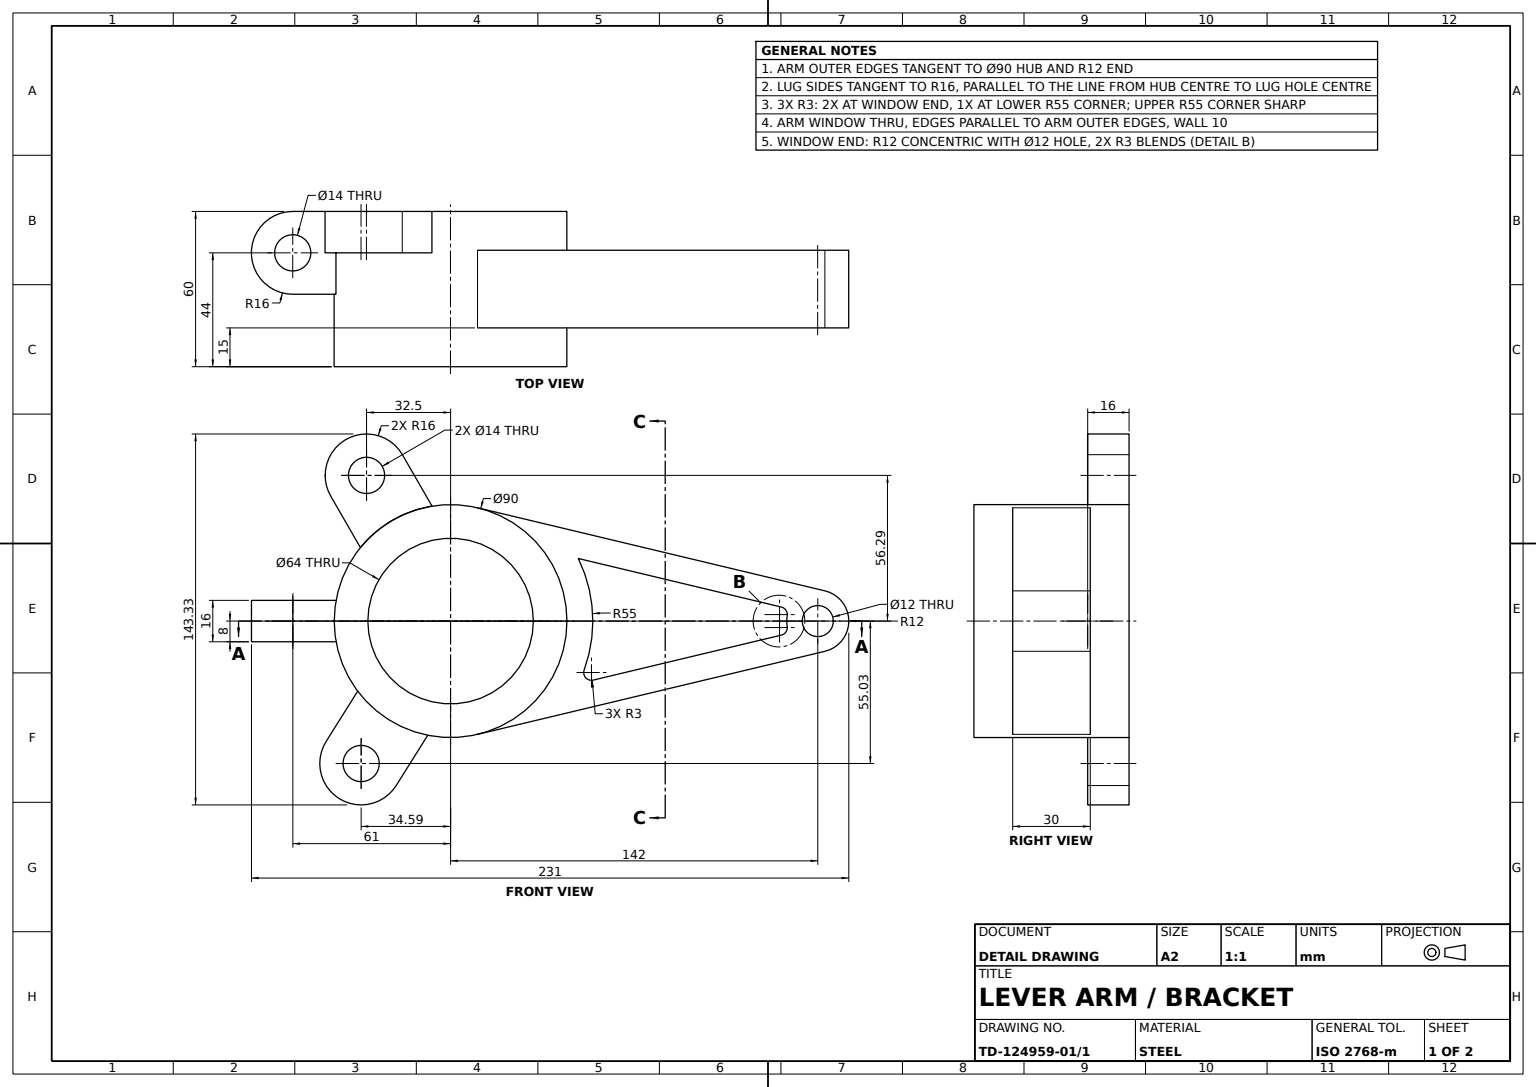
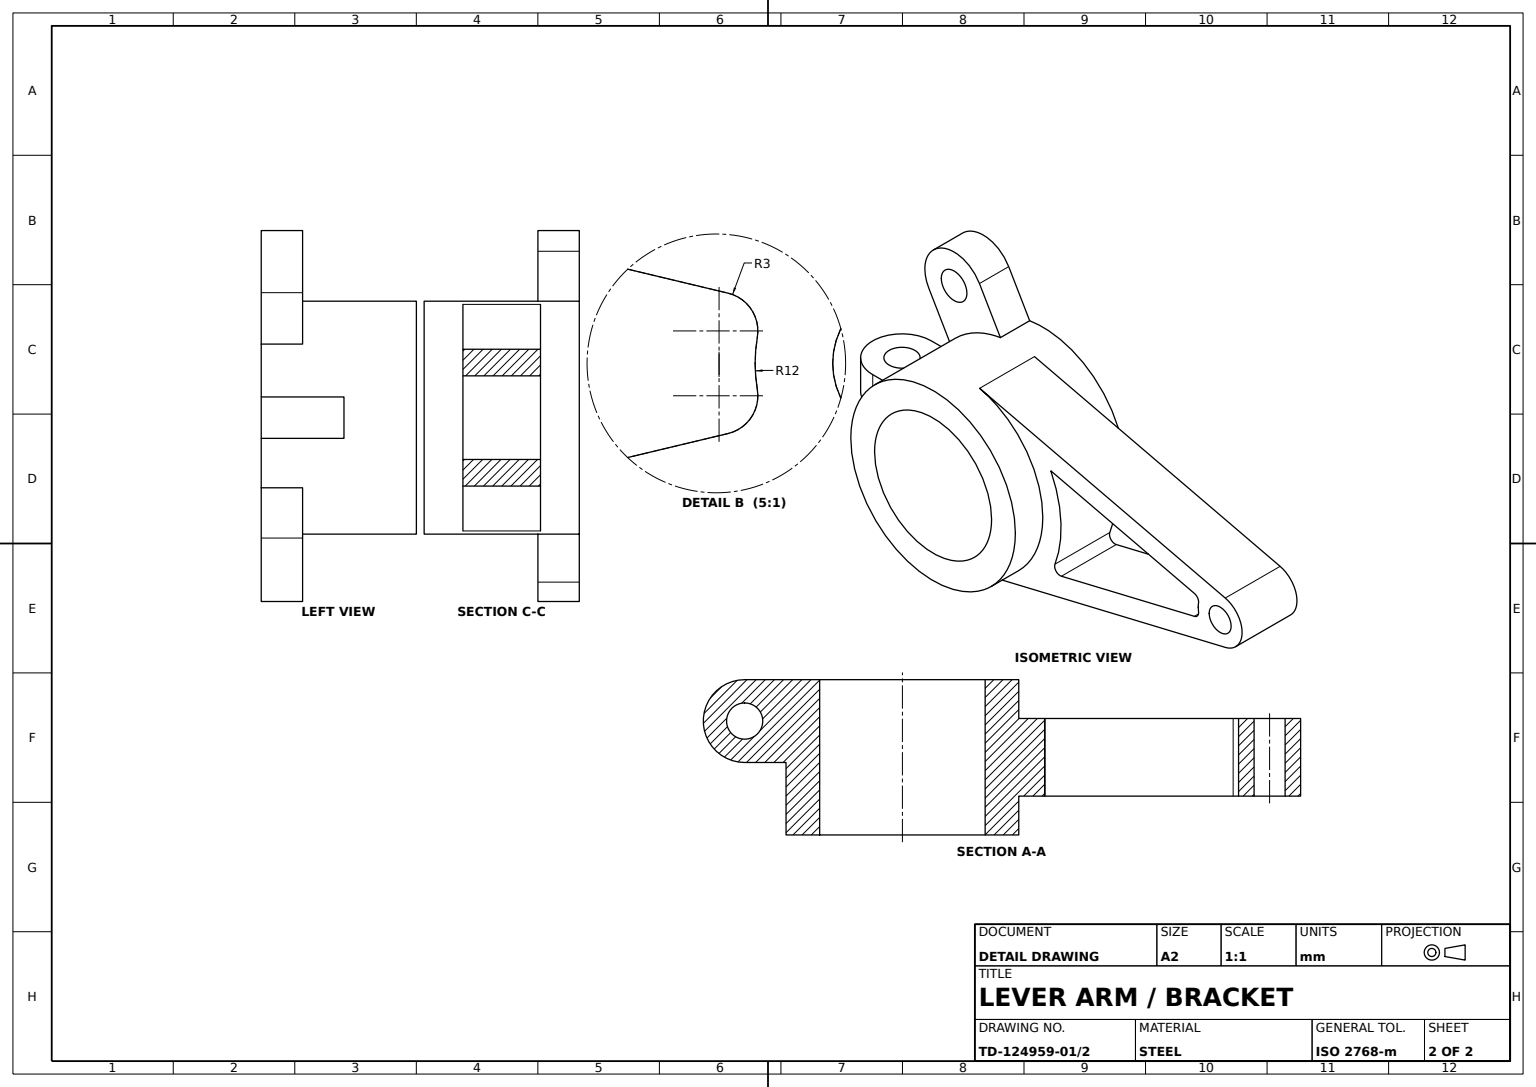
SolidWorks part; units mm, degrees
material "Plain Carbon Steel"
ref_plane "Front Plane" through (0, 0, 0) normal (0, 0, 1) x (1, 0, 0)
ref_plane "Top Plane" through (0, 0, 0) normal (0, 1, 0) x (1, 0, 0)
ref_plane "Right Plane" through (0, 0, 0) normal (1, 0, 0) x (0, 0, -1)
sketch "Hub Profile Ø90xØ64" plane through (0, 0, 0) normal (0, 0, 1) x (1, 0, 0)
  circle A0 centre (0, 0) radius 45
  circle A1 centre (0, 0) radius 32
  dimension "D1" = 90
  dimension "D2" = 64
extrude "Hub Ø90xØ64" add sketch "Hub Profile Ø90xØ64" along normal blind 60
ref_plane "Hub Mid Plane" through (0, 0, 30) normal (0, 0, 1) x (1, 0, 0)
sketch "Arm Web Profile" plane through (0, 0, 30) normal (0, 0, 1) x (1, 0, 0)
  line L0 (0, 0) -> (142, 0) construction
  line L1 (10.4577, 43.768) -> (144.7887, 11.6715)
  line L2 (10.4577, -43.768) -> (144.7887, -11.6715)
  line L3 (49.3986, 24.1821) -> (127.9079, 5.4234)
  line L5 (55.183, -22.8) -> (127.9079, -5.4234)
  line L6 (8.1338, 34.0418) -> (142.4648, 1.9452) construction
  arc A0 (130.1686, 2.0044) -> (130.1686, -2.0044) centre (142, 0) ccw
  circle A1 centre (142, 0) radius 6
  circle A2 centre (0, 0) radius 45 construction
  arc A3 (10.4577, -43.768) -> (10.4577, 43.768) centre (0, 0) ccw
  arc A4 (51.6675, -18.8538) -> (49.3986, 24.1821) centre (0, 0) ccw
  arc A7 (55.183, 22.8) -> (51.6675, 18.8538) centre (54.4858, 19.8822) ccw
  arc A8 (51.6675, -18.8538) -> (55.183, -22.8) centre (54.4858, -19.8822) ccw
  arc A9 (130.1686, 2.0044) -> (127.9079, 5.4234) centre (127.2107, 2.5055) ccw
  arc A10 (127.9079, -5.4234) -> (130.1686, -2.0044) centre (127.2107, -2.5055) ccw
  arc A11 (144.7887, -11.6715) -> (144.7887, 11.6715) centre (142, 0) ccw
  point P20 (8.1338, -34.0418)
  point P21 (142.4648, -1.9452)
  dimension "D1" = 24
  dimension "D2" = 12
  dimension "D4" = 110
  dimension "D5" = 35
  dimension "D6" = 55.183
  dimension "D7" = 3
  dimension "D8" = 3
  dimension "D11" = 3
  dimension "D12" = 3
  dimension "D3" = 142
  dimension "D9" = 127.9079
  dimension "D10" = 22.8
extrude "Webbed Arm" add sketch "Arm Web Profile" along normal mid plane 30 contours L2 A11 L1 A3 A1 A10 L5 A8 A4 L3 A9 A0
ref_plane "Plane3" through (0, 0, 60) normal (0, 0, 1) x (1, 0, 0)
ref_plane "Lug Sketch Plane" through (0, 0, 0) normal (0, 0, 1) x (1, 0, 0)
sketch "Lug A Profile" plane through (0, 0, 0) normal (0, 0, 1) x (1, 0, 0)
  line L0 (0, 0) -> (-61.0486, -56.2781) construction
  line L1 (0, 0) -> (0, 79.901) construction
  line L2 (0, 0) -> (-32.5, 56.2917) construction
  line L4 (-34.8861, 28.4246) -> (-46.3564, 48.2917)
  line L5 (-7.1733, 44.4246) -> (-18.6436, 64.2917)
  line L6 (-13.8564, -8) -> (-46.3564, 48.2917) construction
  arc A0 (-7.1733, 44.4246) -> (-34.8861, 28.4246) centre (0, 0) ccw
  arc A1 (-18.6436, 64.2917) -> (-46.3564, 48.2917) centre (-32.5, 56.2917) ccw
  circle A2 centre (-32.5, 56.2917) radius 7
  point P7 (13.8564, 8)
  dimension "D2" = 90
  dimension "D4" = 16
  dimension "D5" = 14
  dimension "D1" = 30
  dimension "D3" = 65
  dimension "D6" = 19.8671
  dimension "D7" = 83.0311
  dimension "D8" = 47.328
extrude "Lug A 30deg" add sketch "Lug A Profile" along normal blind 16
sketch "Lug B Profile" plane through (0, 0, 0) normal (0, 0, 1) x (1, 0, 0)
  line L0 (0, 0) -> (-34.5873, -55.0338) construction
  line L1 (0, 0) -> (-2.4083, -64.1987) construction
  line L2 (-35.9272, -27.0968) -> (-48.1341, -46.52)
  line L3 (-8.8336, -44.1244) -> (-21.0406, -63.5476)
  line L5 (-13.5468, 8.5138) -> (-48.1341, -46.52) construction
  line L6 (13.5468, -8.5138) -> (-21.0406, -63.5476) construction
  arc A0 (-48.1341, -46.52) -> (-21.0406, -63.5476) centre (-34.5873, -55.0338) ccw
  circle A1 centre (-34.5873, -55.0338) radius 7
  arc A2 (-35.9272, -27.0968) -> (-1.6869, -44.9684) centre (0, 0) ccw
  dimension "D3" = 32
  dimension "D4" = 14
  dimension "D5" = 90
  dimension "D6" = 1.6869
  dimension "D1" = 30
  dimension "D2" = 65
extrude "Lug B 30deg" add sketch "Lug B Profile" along normal blind 16 contours A2 L2 A0 L3 A1
ref_plane "Lug Boss Sketch Plane" through (0, 0, 0) normal (0, 1, 0) x (1, 0, 0)
sketch "Lug Boss Profile" plane through (0, 0, 0) normal (0, 1, 0) x (1, 0, 0)
  line L0 (-45, -60) -> (-45, 0) construction
  line L3 (-18.6436, 0) -> (-48.5, 0) construction
  line L4 (-45, 0) -> (-45, -60) construction
  line L5 (-45, 0) -> (-45, -16) construction
  line L6 (-45, -16) -> (-61, -16) construction
  line L7 (-61, 0) -> (-45, 0)
  line L9 (-61, -32) -> (-45, -32)
  line L11 (-45, 0) -> (-39.0531, 0)
  line L12 (-39.0531, 0) -> (-39.0531, -32)
  line L13 (-39.0531, -32) -> (-45, -32)
  arc A0 (-61, 0) -> (-61, -32) centre (-61, -16) ccw
  dimension "D1" = 32
  dimension "D2" = 5.9469
extrude "Lug Boss" add sketch "Lug Boss Profile" along normal mid plane 16
sketch "Lug Hole Profile" plane through (0, 8, 0) normal (0, 1, 0) x (1, 0, 0)
  circle A0 centre (-61, -16) radius 7
  dimension "D1" = 14
extrude "Lug Through Hole" cut sketch "Lug Hole Profile" against normal blind 16
